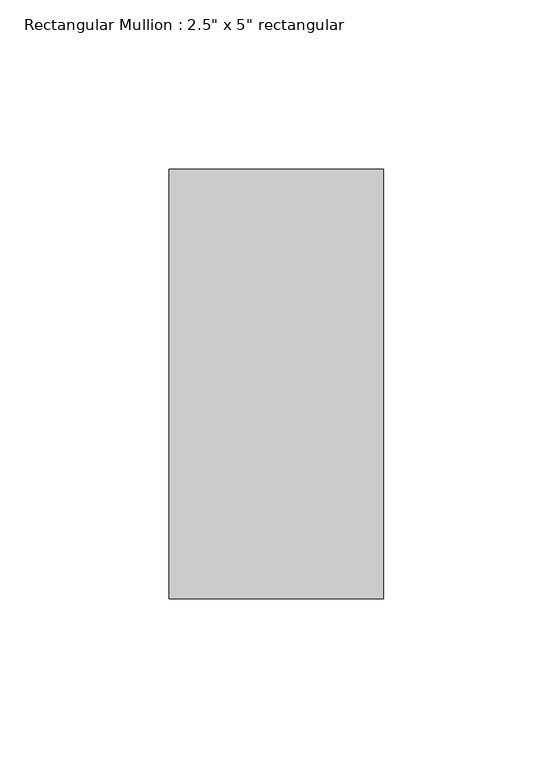
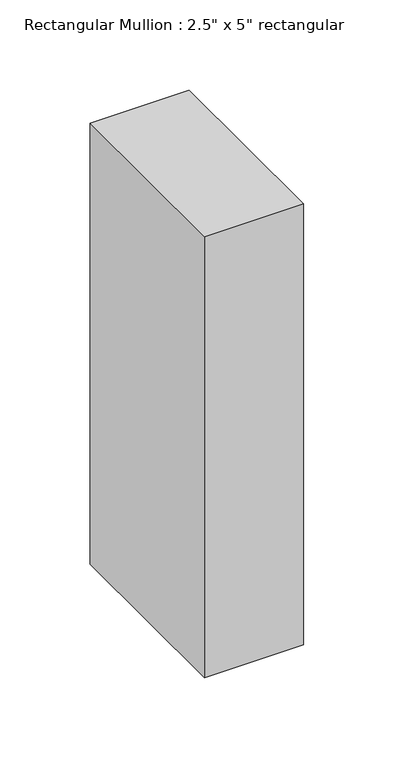
"""IFC4 building model written with IfcOpenShell, lengths in millimetres: member geometry."""

from ifc_helpers import new_model, si_unit, frame, origin, place, context, project, spatial, polyline, outline, extrude, source, transform, mapped, element, save


def member_8199a1f0(model_context):
    return source(origin(), model_context, "Body", "SweptSolid", [
        extrude(outline(polyline([(0.0, 63.5), (0.0, -63.5), (-63.5, -63.5), (-63.5, 63.5), (0.0, 63.5)])), frame((0.0, 0.0, -298.45), z_axis=(0.0, 0.0, 1.0), x_axis=(1.0, 0.0, 0.0)), (0.0, 0.0, 1.0), 298.45),
    ])


if __name__ == "__main__":
    model = new_model("IFC4")
    model_context = context("Model", 3, world=origin())
    ifc_project = project(units=[si_unit("LENGTHUNIT", "METRE", prefix="MILLI")], contexts=[model_context])
    site = spatial("IfcSite", under=ifc_project)
    building = spatial("IfcBuilding", under=site)
    placement = place(None, origin())
    member_shape = member_8199a1f0(model_context)
    element("IfcMember", 1, ObjectType="Rectangular Mullion : 2.5\" x 5\" rectangular", at=placement, inside=building, context=model_context, shape_type="MappedRepresentation", body=[
        mapped(member_shape, transform((0.0, 0.0, 0.0), x_axis=(1.0, 0.0, 0.0), y_axis=(0.0, 1.0, 0.0), z_axis=(0.0, 0.0, 1.0))),
    ])
    save(model, "model.ifc")

# Revit data of these elements
# Type "Rectangular Mullion : 2.5\" x 5\" rectangular"
#   built-in parameter 1007304 = 0.416667 (stored number, unit not read)
#   built-in parameter 1007301 = 0.104167 (stored number, unit not read)
#   built-in parameter 1007300 = 0.104167 (stored number, unit not read)
# Element 1 (IfcMember, "Rectangular Mullion : 2.5\" x 5\" rectangular")
#   Materials on its faces: "Aluminum"
# Materials
#   "Aluminum": class "Metal", colour RGB 247 247 247, transparency 0, Description = "Aluminum 6061", Cost = 0
